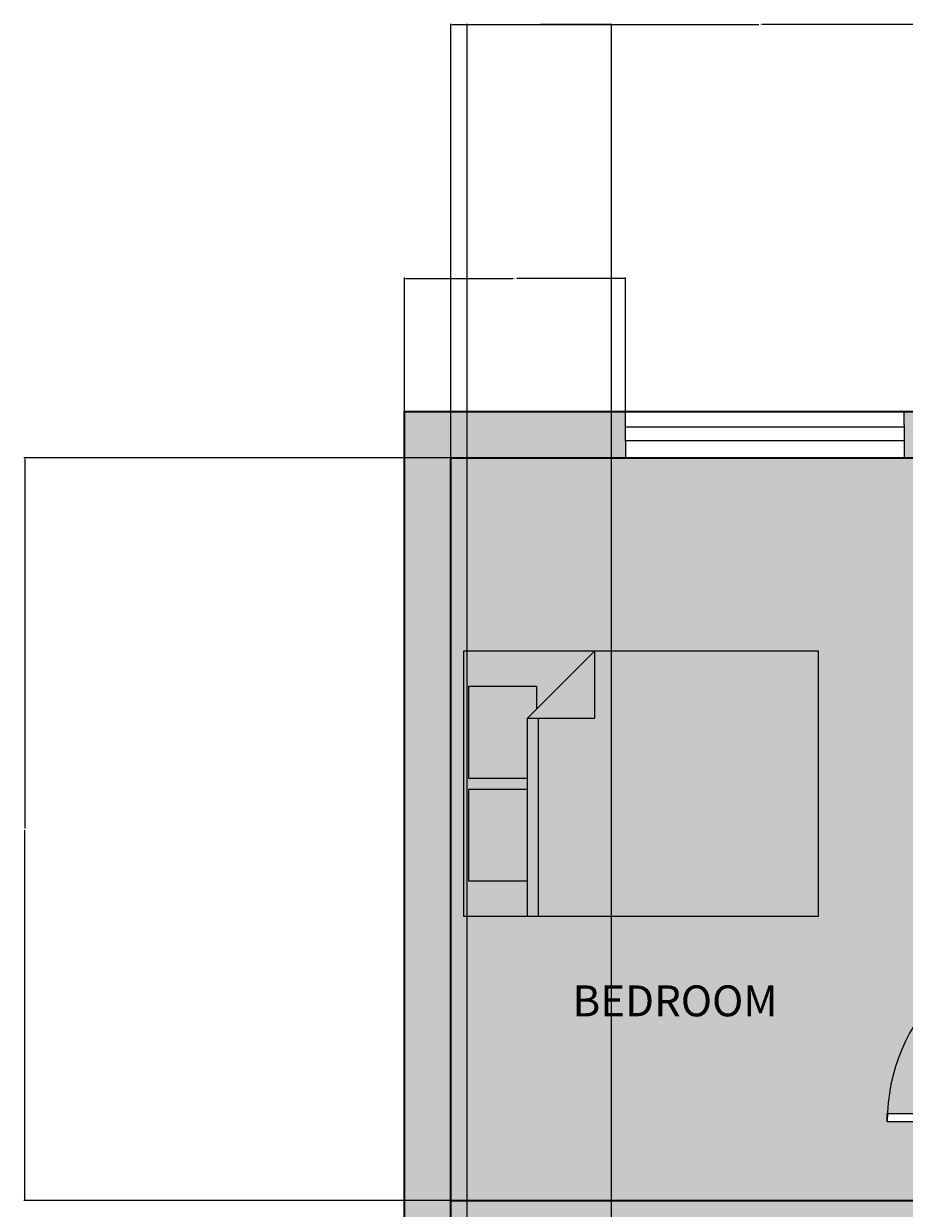
# Model space of a CAD drawing. Units: inches. Extents: x 3024 to 3952, y 1308 to 1863.
# Tile 22 of 29: x 3024 to 3195, y 1633 to 1863. Entities that reach past the tile are written whole.
import ezdxf

# ---------------------------------------------------------------- set-up
doc = ezdxf.new("R2010")
doc.units = ezdxf.units.IN
for name, color, linetype, lineweight in [('A-ANNO-DIMS', 2, 'Continuous', 18), ('A-AREA-IDEN', 7, 'Continuous', 18), ('A-DOOR', 4, 'Continuous', 18), ('A-FLOR-TILE-PATT', 7, 'Continuous', 13), ('A-FURN', 8, 'Continuous', 18), ('A-FURN-PATT', 9, 'Continuous', 13), ('A-GLAZ', 4, 'Continuous', 18), ('A-WALL', 7, 'Continuous', 35)]:
    doc.layers.add(name, color=color, linetype=linetype, lineweight=lineweight)
doc.layers.add('A-FLOR-PATT', color=254, linetype='Continuous', lineweight=13, true_color=0xfeeab9)
doc.layers.add('A-WALL-PATT', color=254, linetype='Continuous', lineweight=13, true_color=0xcecce6)
doc.styles.get("Standard").update_dxf_attribs({"font": 'arial.ttf'})
doc.dimstyles.get("Standard").update_dxf_attribs({"dimtxt": 0.18, "dimasz": 0.18, "dimexe": 0.18, "dimexo": 0.0625, "dimgap": 0.09, "dimtad": 0, "dimtih": 1, "dimtoh": 1, "dimdec": 4, "dimzin": 0, "dimdsep": 46, "dimtxsty": 'Standard', "dimcen": 0.09, "dimadec": 0, "dimazin": 0, "dimtfac": 1, "dimtdec": 4, "dimtofl": 0, "dimtmove": 0, "dimatfit": 3, "dimfxl": 1, "dimtolj": 1, "dimtzin": 0, "dimarcsym": 0})

# ---------------------------------------------------------------- blocks, each defined once
blk = doc.blocks.new('*U2')
for p, q in [((0, 0), (0, -6)), ((40, 0), (40, -6))]:
    blk.add_line(p, q)
blk.add_lwpolyline([(0, 0), (0, 40), (1.75, 40), (1.75, 0)], close=True)
blk.add_arc((0, 0), 40, 0, 90)
blk = doc.blocks.new('Bed - Queen')
for p, q in [((0, -80.00003), (0, 0)), ((0, 0), (59.99999, 0)), ((59.99999, 0), (59.99999, -80.00003)), ((7.99999, -1.2), (28.79998, -1.2)), ((7.99999, -14.4), (7.99999, -1.2)), ((28.79998, -1.2), (28.79998, -14.4)), ((31.19999, -1.2), (51.99999, -1.2)), ((31.19999, -14.4), (31.19999, -1.2)), ((51.99999, -1.2), (51.99999, -16.4)), ((0, -14.4), (44.8, -14.4)), ((59.99999, -29.6), (44.8, -14.4)), ((44.8, -14.4), (44.8, -29.6)), ((44.8, -16.8), (0, -16.8)), ((51.99999, -16.4), (46.79936, -16.4)), ((44.8, -29.6), (59.99999, -29.6)), ((59.99999, -80.00003), (0, -80.00003))]:
    blk.add_line(p, q)
blk = doc.blocks.new('WIN-BEDROOM-54IN')
for p, q in [((0, 5.99), (0, 9)), ((54.08, 6.41), (54.08, 9)), ((54.08, 6.41), (54.08, 5.99)), ((0, 3.28), (0, 0)), ((54.08, 3.69), (54.08, 0))]:
    blk.add_line(p, q)
blk.add_lwpolyline([(0, 5.99), (54.08, 5.99), (54.08, 3.28), (0, 3.28)], close=True)
blk = doc.blocks.new('*D38')
at = {"layer": 'A-ANNO-DIMS', "color": 0, "lineweight": -2, "transparency": 16777216}
for p, q in [((3106.76, 1778.67), (3106.76, 1862.78)), ((3226.76, 1778.67), (3226.76, 1862.78)), ((3106.94, 1862.6), (3166.48, 1862.6)), ((3226.58, 1862.6), (3167.04, 1862.6))]:
    blk.add_line(p, q, dxfattribs=at)
at = {"layer": 'A-ANNO-DIMS', "color": 0, "transparency": 16777216}
for points in [[(3106.94, 1862.63), (3106.94, 1862.57), (3106.76, 1862.6)], [(3226.58, 1862.63), (3226.58, 1862.57), (3226.76, 1862.6)]]:
    blk.add_solid(points, dxfattribs=at)
at = {"layer": 'Defpoints', "color": 0, "transparency": 16777216}
for p in [(3226.76, 1862.6), (3106.76, 1778.61), (3226.76, 1778.61)]:
    blk.add_point(p, dxfattribs=at)
at = {"layer": 'A-ANNO-DIMS', "color": 0, "transparency": 16777216, "insert": (3166.76, 1862.6), "char_height": 0.18, "attachment_point": 5}
blk.add_mtext('\\A1;120', dxfattribs=at)
blk = doc.blocks.new('*D42')
at = {"layer": 'A-ANNO-DIMS', "color": 0, "lineweight": -2, "transparency": 16777216}
for p, q in [((3106.7, 1778.61), (3023.95, 1778.61)), ((3024.13, 1778.43), (3024.13, 1706.79)), ((3024.13, 1634.79), (3024.13, 1706.43)), ((3106.7, 1634.61), (3023.95, 1634.61))]:
    blk.add_line(p, q, dxfattribs=at)
at = {"layer": 'A-ANNO-DIMS', "color": 0, "transparency": 16777216}
for points in [[(3024.1, 1778.43), (3024.16, 1778.43), (3024.13, 1778.61)], [(3024.1, 1634.79), (3024.16, 1634.79), (3024.13, 1634.61)]]:
    blk.add_solid(points, dxfattribs=at)
at = {"layer": 'Defpoints', "color": 0, "transparency": 16777216}
for p in [(3106.76, 1778.61), (3024.13, 1634.61), (3106.76, 1634.61)]:
    blk.add_point(p, dxfattribs=at)
at = {"layer": 'A-ANNO-DIMS', "color": 0, "transparency": 16777216, "insert": (3024.13, 1706.61), "char_height": 0.18, "attachment_point": 5}
blk.add_mtext('\\A1;144', dxfattribs=at)
blk = doc.blocks.new('*D71')
at = {"layer": 'A-ANNO-DIMS', "color": 0, "lineweight": -2, "transparency": 16777216}
for p, q in [((3097.76, 1787.67), (3097.76, 1813.56)), ((3097.94, 1813.38), (3118.78, 1813.38)), ((3140.42, 1813.38), (3119.58, 1813.38)), ((3140.6, 1787.67), (3140.6, 1813.56))]:
    blk.add_line(p, q, dxfattribs=at)
at = {"layer": 'A-ANNO-DIMS', "color": 0, "transparency": 16777216}
for points in [[(3097.94, 1813.41), (3097.94, 1813.35), (3097.76, 1813.38)], [(3140.42, 1813.41), (3140.42, 1813.35), (3140.6, 1813.38)]]:
    blk.add_solid(points, dxfattribs=at)
at = {"layer": 'Defpoints', "color": 0, "transparency": 16777216}
for p in [(3140.6, 1813.38), (3097.76, 1787.61), (3140.6, 1787.61)]:
    blk.add_point(p, dxfattribs=at)
at = {"layer": 'A-ANNO-DIMS', "color": 0, "transparency": 16777216, "insert": (3119.18, 1813.38), "char_height": 0.18, "attachment_point": 5}
blk.add_mtext('\\A1;42.83', dxfattribs=at)
blk = doc.blocks.new('*D80')
at = {"layer": 'A-ANNO-DIMS', "color": 0, "lineweight": -2, "transparency": 16777216}
for p, q in [((3109.9, 1617.34), (3109.9, 1862.78)), ((3137.9, 1606.84), (3137.9, 1862.78)), ((3110.08, 1862.6), (3123.68, 1862.6)), ((3137.72, 1862.6), (3124.12, 1862.6))]:
    blk.add_line(p, q, dxfattribs=at)
at = {"layer": 'A-ANNO-DIMS', "color": 0, "transparency": 16777216}
for points in [[(3110.08, 1862.63), (3110.08, 1862.57), (3109.9, 1862.6)], [(3137.72, 1862.63), (3137.72, 1862.57), (3137.9, 1862.6)]]:
    blk.add_solid(points, dxfattribs=at)
at = {"layer": 'Defpoints', "color": 0, "transparency": 16777216}
for p in [(3137.9, 1862.6), (3109.9, 1617.28), (3137.9, 1606.78)]:
    blk.add_point(p, dxfattribs=at)
at = {"layer": 'A-ANNO-DIMS', "color": 0, "transparency": 16777216, "insert": (3123.9, 1862.6), "char_height": 0.18, "attachment_point": 5}
blk.add_mtext('\\A1;28', dxfattribs=at)

msp = doc.modelspace()

# ---------------------------------------------------------------- hatches: boundary and pattern name
at = {"layer": 'A-FLOR-PATT', "transparency": 33554528}
h = msp.add_hatch(color=256, dxfattribs=at)
h.dxf.hatch_style = 1
h.paths.add_polyline_path([(3460.764, 1688.6064), (3412.764, 1688.6064), (3412.764, 1694.6064), (3460.764, 1694.6064), (3460.764, 1778.6064), (3406.764, 1778.6064), (3406.764, 1759.9514), (3318.2981, 1759.9514), (3318.2981, 1658.6064), (3322.5356, 1658.6064), (3322.5356, 1652.6064), (3292.764, 1652.6064), (3292.764, 1778.6064), (3106.764, 1778.6064), (3106.764, 1628.6064), (3172.764, 1628.6064), (3172.764, 1532.6064), (3166.764, 1532.6064), (3166.764, 1628.6064), (3106.764, 1628.6064), (3106.764, 1356.8452), (3202.812, 1356.8452), (3202.812, 1354.2534), (3202.812, 1353.8388), (3202.812, 1351.1212), (3202.812, 1347.8452), (3277.764, 1347.8452), (3277.764, 1353.8452), (3277.764, 1356.8452), (3277.764, 1442.6064), (3460.764, 1442.6064)])
h.paths.add_polyline_path([(3216.238, 1527.2064), (3216.238, 1491.2064), (3214.663, 1491.2064), (3214.663, 1491.2409, -0.39662236), (3180.243, 1526.6064), (3163.0285, 1526.6064), (3163.0285, 1531.1064), (3161.716, 1531.1064), (3161.716, 1561.1064), (3163.0285, 1561.1064), (3163.0285, 1531.1064), (3163.0285, 1526.6064), (3180.243, 1526.6064, 0.39662236), (3214.663, 1491.2409), (3214.663, 1527.2064)], flags=16)
h.paths.add_polyline_path([(3227.364, 1649.8972), (3191.364, 1649.8972), (3191.364, 1651.4722), (3227.364, 1651.4722)], flags=16)
h.paths.add_polyline_path([(3323.1172, 1606.7362), (3323.8545, 1606.8514), (3323.8545, 1594.8241), (3323.1172, 1594.9393)], flags=16)
h.paths.add_polyline_path([(3324.2232, 1606.909), (3330.1216, 1607.8307), (3330.1216, 1614.1093), (3339.3495, 1614.1093), (3340.2711, 1620.0078), (3352.4136, 1620.0078), (3353.3353, 1614.1093), (3359.9941, 1614.1093), (3360.9157, 1620.0078), (3373.0582, 1620.0078), (3373.9799, 1614.1093), (3383.2077, 1614.1093), (3383.2077, 1607.8307), (3389.1062, 1606.909), (3389.1062, 1594.7665), (3383.2077, 1593.8449), (3383.2077, 1587.5663), (3373.9799, 1587.5663), (3373.0583, 1581.6678), (3360.9157, 1581.6678), (3359.9941, 1587.5663), (3353.3353, 1587.5663), (3352.4136, 1581.6678), (3340.2711, 1581.6678), (3339.3495, 1587.5663), (3330.1216, 1587.5663), (3330.1216, 1593.8449), (3324.2232, 1594.7665)], flags=16)
h.paths.add_polyline_path([(3236.1584, 1693.1064), (3236.1584, 1723.1064), (3237.4709, 1723.1064), (3237.4709, 1693.1064)], flags=16)
h.paths.add_polyline_path([(3373.2158, 1600.6847), (3373.7965, 1600.7303), (3374.3268, 1600.7874), (3374.8132, 1600.8531), (3375.2621, 1600.9247), (3375.6801, 1600.9991), (3376.0736, 1601.0735), (3376.6855, 1601.19), (3377.366, 1601.3023), (3378.0667, 1601.3814), (3378.8026, 1601.4123), (3379.5865, 1601.3839), (3380.4537, 1601.2948), (3381.301, 1601.1717), (3382.0317, 1601.0433), (3382.4398, 1600.9607), (3382.6252, 1600.9201), (3382.919, 1600.8507), (3382.9044, 1600.8531), (3382.842, 1600.8678), (3382.7541, 1600.8896), (3382.6252, 1600.9201), (3382.4398, 1600.9607), (3382.1868, 1601.0119), (3381.8738, 1601.0711), (3381.5125, 1601.1346), (3381.1149, 1601.1988), (3380.6928, 1601.2601), (3380.2581, 1601.3149), (3379.8226, 1601.3597), (3379.3984, 1601.3908), (3378.9944, 1601.4054), (3378.6092, 1601.4042), (3378.2384, 1601.3886), (3377.8777, 1601.36), (3377.5227, 1601.32), (3377.1691, 1601.2698), (3376.8127, 1601.211), (3376.4491, 1601.145), (3376.0736, 1601.0735), (3375.4177, 1600.9494), (3374.5542, 1600.8119), (3373.5044, 1600.6988)], flags=0)
h.paths.add_polyline_path([(3380.0253, 1596.7351), (3380.499, 1596.6659), (3380.9706, 1596.6119), (3381.4375, 1596.5791), (3381.8971, 1596.5736), (3382.5886, 1596.6167), (3382.7848, 1596.6692), (3382.1465, 1596.5706), (3381.236, 1596.5815), (3380.3199, 1596.6865)], flags=0)
h.paths.add_polyline_path([(3369.6414, 1603.9617), (3370.1589, 1604.0021), (3370.6218, 1604.0539), (3371.0335, 1604.1173), (3371.3978, 1604.1921), (3371.7181, 1604.2785), (3371.9984, 1604.3761), (3372.2441, 1604.483), (3372.4611, 1604.5972), (3372.655, 1604.7163), (3372.8317, 1604.8384), (3372.9968, 1604.9611), (3373.3703, 1605.2455), (3373.8426, 1605.5328), (3374.4624, 1605.7539), (3375.1058, 1605.8302), (3375.7221, 1605.8261), (3376.4109, 1605.76), (3377.1534, 1605.6376), (3377.8945, 1605.473), (3378.1382, 1605.409), (3377.7394, 1605.5074), (3377.3509, 1605.5937), (3376.9704, 1605.6677), (3376.5999, 1605.7288), (3376.2417, 1605.7762), (3375.8979, 1605.8092), (3375.5707, 1605.8271), (3375.2621, 1605.8291), (3374.9745, 1605.8146), (3374.7092, 1605.7832), (3374.4647, 1605.7359), (3374.239, 1605.6742), (3374.0298, 1605.5996), (3373.835, 1605.5134), (3373.6525, 1605.4171), (3373.4801, 1605.3123), (3373.3156, 1605.2002), (3373.1562, 1605.0825), (3372.7603, 1604.781), (3372.236, 1604.4588), (3371.5738, 1604.2283), (3370.8493, 1604.0794), (3369.9262, 1603.976)], flags=0)
h.paths.add_polyline_path([(3366.7533, 1606.5832), (3367.1713, 1606.5519), (3367.5378, 1606.5374), (3367.8568, 1606.5394), (3368.1325, 1606.5573), (3368.3694, 1606.5903), (3368.5717, 1606.6377), (3368.7438, 1606.6988), (3368.89, 1606.7728), (3369.0146, 1606.8591), (3369.121, 1606.9568), (3369.2094, 1607.0646), (3369.2792, 1607.181), (3369.3295, 1607.3046), (3369.3596, 1607.4339), (3369.3688, 1607.5676), (3369.3565, 1607.7042), (3369.3218, 1607.8422), (3369.2649, 1607.9804), (3369.1893, 1608.1187), (3369.0993, 1608.2569), (3368.9992, 1608.3952), (3368.8934, 1608.5334), (3368.7861, 1608.6717), (3368.6817, 1608.8099), (3368.4212, 1609.1804), (3368.2685, 1609.7106), (3368.4883, 1610.1814), (3369.0537, 1610.4604), (3369.6717, 1610.5097), (3370.2812, 1610.3612), (3370.4805, 1610.2968), (3370.1882, 1610.3839), (3369.9284, 1610.4472), (3369.6905, 1610.4842), (3369.4662, 1610.4933), (3369.2555, 1610.4765), (3369.0608, 1610.4367), (3368.884, 1610.3767), (3368.7274, 1610.2994), (3368.5931, 1610.2077), (3368.4833, 1610.1045), (3368.4002, 1609.9927), (3368.3451, 1609.8747), (3368.3166, 1609.7517), (3368.3127, 1609.6244), (3368.331, 1609.4935), (3368.3696, 1609.3597), (3368.4261, 1609.2237), (3368.4985, 1609.0863), (3368.5845, 1608.9482), (3368.6817, 1608.8099), (3368.7861, 1608.6717), (3368.8934, 1608.5334), (3368.9992, 1608.3952), (3369.0993, 1608.2569), (3369.3398, 1607.8876), (3369.3941, 1607.2896), (3368.9774, 1606.7817), (3368.3928, 1606.5742), (3367.7162, 1606.5303), (3367.0044, 1606.5585)], flags=0)
h.paths.add_polyline_path([(3362.1859, 1610.2589), (3362.5478, 1610.2845), (3362.8348, 1610.3275), (3363.0585, 1610.3863), (3363.2303, 1610.4595), (3363.3619, 1610.5457), (3363.463, 1610.6432), (3363.5376, 1610.7502), (3363.5876, 1610.8643), (3363.6153, 1610.9834), (3363.6229, 1611.1055), (3363.6125, 1611.2283), (3363.5861, 1611.3496), (3363.5462, 1611.4673), (3363.4949, 1611.5797), (3363.4358, 1611.6871), (3363.3723, 1611.7902), (3363.3081, 1611.8897), (3363.2468, 1611.9863), (3363.192, 1612.0808), (3363.0258, 1612.4261), (3363.3371, 1612.8672), (3363.9008, 1612.9782), (3364.4822, 1612.9641), (3365.1098, 1612.9074), (3365.328, 1612.8805), (3364.9615, 1612.9208), (3364.6426, 1612.9496), (3364.3668, 1612.9669), (3364.1299, 1612.9726), (3363.9276, 1612.9669), (3363.7555, 1612.9496), (3363.6093, 1612.9208), (3363.4848, 1612.8805), (3363.3782, 1612.8289), (3363.2889, 1612.7672), (3363.2169, 1612.6969), (3363.1622, 1612.6193), (3363.1247, 1612.5361), (3363.1046, 1612.4484), (3363.1017, 1612.358), (3363.1161, 1612.266), (3363.1472, 1612.1738), (3363.192, 1612.0808), (3363.2468, 1611.9863), (3363.3081, 1611.8897), (3363.3723, 1611.7902), (3363.4358, 1611.6871), (3363.6363, 1611.323), (3363.5979, 1610.7003), (3363.0863, 1610.3651), (3362.3983, 1610.2622)], flags=0)
h.paths.add_polyline_path([(3352.356, 1581.2991), (3352.2408, 1580.5618), (3340.4439, 1580.5618), (3340.3287, 1581.2991)], flags=16)
h.paths.add_polyline_path([(3340.4439, 1621.1137), (3352.2408, 1621.1137), (3352.356, 1620.3764), (3340.3287, 1620.3764)], flags=16)
h.paths.add_polyline_path([(3278.4282, 1504.7424), (3290.3831, 1504.7424), (3290.3831, 1502.7499), (3291.0473, 1502.7499), (3291.0473, 1494.7799), (3290.3831, 1494.7799), (3290.3831, 1494.1158), (3291.0473, 1494.1158), (3291.0473, 1486.1458), (3290.3831, 1486.1458), (3290.3831, 1484.1533), (3291.0473, 1484.1533), (3291.0473, 1483.4892, -0.09090909), (3291.0473, 1468.8776), (3291.0473, 1468.2135), (3290.3831, 1468.2135), (3290.3831, 1464.8926), (3278.4282, 1464.8926), (3278.4282, 1472.8626), (3277.764, 1473.5268), (3277.764, 1478.84), (3278.4282, 1479.5042)], flags=16)
h.paths.add_polyline_path([(3278.7603, 1504.4103), (3290.051, 1504.4103), (3290.051, 1465.2247), (3278.7603, 1465.2247)], flags=0)
h.paths.add_polyline_path([(3123.904, 1600.7821), (3117.9039, 1602.7821), (3117.9039, 1599.7821), (3119.4039, 1599.7821), (3119.4039, 1596.7821), (3118.4039, 1596.7821), (3118.4039, 1598.7821), (3117.9039, 1598.7821), (3117.9039, 1596.2821), (3109.9039, 1596.2821), (3109.9039, 1617.2821), (3117.9039, 1617.2821), (3117.9039, 1610.7821), (3123.9038, 1612.7821, -0.70257121), (3137.9039, 1606.7822, -0.70256205)], flags=16)
h.paths.add_polyline_path([(3123.9039, 1602.7822), (3123.9039, 1610.7822, -0.73453329), (3136.9039, 1606.7822, -0.73452973)], flags=0)
h.paths.add_polyline_path([(3177.972, 1689.6473), (3109.2405, 1689.6473), (3109.2405, 1741.1959), (3177.972, 1741.1959)], flags=16)
h.paths.add_polyline_path([(3373.0006, 1581.2991), (3372.8854, 1580.5618), (3361.0885, 1580.5618), (3360.9733, 1581.2991)], flags=16)
h.paths.add_polyline_path([(3361.0885, 1621.1137), (3372.8854, 1621.1137), (3373.0006, 1620.3764), (3360.9733, 1620.3764)], flags=16)
h.paths.add_polyline_path([(3116.9039, 1598.2821, -0.41421356), (3116.1539, 1597.2821), (3111.9039, 1597.2821, -0.41421356), (3110.9039, 1598.0321), (3110.9039, 1615.2821, -0.41421356), (3111.6539, 1616.2821), (3115.9039, 1616.2821, -0.41421356), (3116.9039, 1615.5321)], flags=0)
h.paths.add_polyline_path([(3121.6122, 1728.1369), (3121.6122, 1696.5205), (3110.2715, 1696.5205), (3110.2715, 1714.3906), (3121.6122, 1714.3906), (3121.6122, 1716.4526), (3110.2715, 1716.4526), (3110.2715, 1734.3228), (3123.3304, 1734.3228), (3123.3304, 1729.8552), (3134.6711, 1741.1959), (3134.6711, 1728.1369)], flags=0)
h.paths.add_polyline_path([(3389.4748, 1606.8514), (3390.2122, 1606.7362), (3390.2122, 1594.9393), (3389.4748, 1594.8241)], flags=16)
h.paths.add_polyline_path([(3257.6842, 1762.8281), (3259.6842, 1768.8281), (3256.6842, 1768.8281), (3256.6842, 1767.3281), (3253.6842, 1767.3281), (3253.6842, 1768.3281), (3255.6842, 1768.3281), (3255.6842, 1768.8281), (3253.1842, 1768.8281), (3253.1842, 1776.8281), (3274.1842, 1776.8281), (3274.1842, 1768.8281), (3267.6842, 1768.8281), (3269.6842, 1762.8282, -0.70257121), (3263.6843, 1748.8282, -0.70256205)], flags=16)
h.paths.add_polyline_path([(3259.6842, 1762.8281), (3267.6843, 1762.8281, -0.73453329), (3263.6842, 1749.8282, -0.73452973)], flags=0)
h.paths.add_polyline_path([(3411.264, 1715.6064), (3411.264, 1716.9189), (3441.264, 1716.9189), (3441.264, 1715.6064)], flags=16)
h.paths.add_polyline_path([(3178.3806, 1449.1876), (3178.3806, 1397.639), (3109.6491, 1397.639), (3109.6491, 1449.1876)], flags=16)
h.paths.add_polyline_path([(3397.1501, 1541.7146), (3419.6183, 1541.7146), (3419.6183, 1496.7783), (3397.1501, 1496.7783)], flags=16)
h.paths.add_polyline_path([(3254.1842, 1770.5781), (3254.1842, 1774.8281, -0.41421356), (3254.9342, 1775.8281), (3272.1842, 1775.8281, -0.41421356), (3273.1842, 1775.0781), (3273.1842, 1770.8281, -0.41421356), (3272.4342, 1769.8281), (3255.1842, 1769.8281, -0.41421356)], flags=0)
h.paths.add_polyline_path([(3403.672, 1500.7601), (3403.6016, 1500.3997), (3403.5328, 1500.0441), (3403.4662, 1499.6867), (3403.4027, 1499.3226), (3403.3464, 1498.9532), (3403.3025, 1498.5811), (3403.2759, 1498.2091), (3403.2714, 1497.8401), (3403.3064, 1497.2813), (3403.3491, 1497.1219), (3403.2689, 1497.6395), (3403.2778, 1498.3719), (3403.3635, 1499.0984), (3403.4889, 1499.8168), (3403.6016, 1500.3997), (3403.672, 1500.7601), (3403.744, 1501.1315), (3403.817, 1501.5205), (3403.891, 1501.9336), (3403.9656, 1502.3769), (3404.0404, 1502.8572), (3404.115, 1503.3786), (3404.2264, 1504.2311), (3404.2571, 1504.5223), (3404.1552, 1503.6598), (3404.0063, 1502.6193), (3403.8604, 1501.7518), (3403.744, 1501.1315)], flags=0)
h.paths.add_polyline_path([(3406.5868, 1505.0416), (3406.6121, 1504.5236), (3406.6492, 1504.0526), (3406.6956, 1503.624), (3406.7491, 1503.2333), (3406.8072, 1502.8759), (3406.8676, 1502.5473), (3406.9281, 1502.243), (3407.0268, 1501.7597), (3407.1416, 1501.1368), (3407.2087, 1500.3904), (3407.1804, 1499.6703), (3407.1078, 1498.9956), (3407.0074, 1498.3199), (3406.8809, 1497.6059), (3406.7403, 1496.9627), (3406.7418, 1496.9824), (3406.7491, 1497.0249), (3406.8229, 1497.3409), (3406.8364, 1497.4025), (3406.878, 1497.6078), (3406.9261, 1497.8614), (3406.9777, 1498.1526), (3407.0298, 1498.4712), (3407.0797, 1498.8068), (3407.1243, 1499.149), (3407.1607, 1499.4874), (3407.1859, 1499.8115), (3407.1978, 1500.1137), (3407.1969, 1500.3962), (3407.1841, 1500.6642), (3407.1609, 1500.9225), (3407.1284, 1501.1761), (3407.0876, 1501.43), (3407.0398, 1501.6891), (3406.9862, 1501.9585), (3406.8832, 1502.4628), (3406.7712, 1503.0713), (3406.6657, 1503.8424), (3406.5924, 1504.7735)], flags=0)
h.paths.add_polyline_path([(3409.2517, 1507.8962), (3409.2752, 1507.4282), (3409.3079, 1507.0076), (3409.3501, 1506.6314), (3409.4015, 1506.2969), (3409.4624, 1506.0009), (3409.5326, 1505.7406), (3409.6119, 1505.5128), (3409.6988, 1505.3131), (3409.7915, 1505.1368), (3409.8883, 1504.9792), (3409.9875, 1504.8356), (3410.0872, 1504.7015), (3410.1859, 1504.572), (3410.4508, 1504.2132), (3410.7205, 1503.6035), (3410.8059, 1502.8824), (3410.7619, 1502.0875), (3410.6122, 1501.2299), (3410.4402, 1500.6169), (3410.2538, 1500.0031), (3410.0536, 1499.3219), (3409.9909, 1499.0812), (3410.1761, 1499.7472), (3410.3596, 1500.3513), (3410.4512, 1500.6561), (3410.5312, 1500.9412), (3410.6013, 1501.226), (3410.6614, 1501.512), (3410.7111, 1501.7964), (3410.7496, 1502.0763), (3410.7764, 1502.3489), (3410.7909, 1502.6114), (3410.7926, 1502.8608), (3410.7808, 1503.0944), (3410.7553, 1503.31), (3410.7169, 1503.5087), (3410.6667, 1503.6921), (3410.6061, 1503.8621), (3410.5361, 1504.0203), (3410.4578, 1504.1686), (3410.3726, 1504.3088), (3410.2815, 1504.4424), (3410.1859, 1504.572), (3410.0872, 1504.7015), (3409.859, 1505.0083), (3409.5943, 1505.5117), (3409.4266, 1506.1336), (3409.324, 1506.8011), (3409.2586, 1507.6407)], flags=0)
h.paths.add_polyline_path([(3411.4914, 1510.5878), (3411.4432, 1510.1586), (3411.4054, 1509.775), (3411.38, 1509.4354), (3411.3681, 1509.1376), (3411.3698, 1508.8784), (3411.3843, 1508.6542), (3411.4112, 1508.4618), (3411.4497, 1508.2974), (3411.4994, 1508.1575), (3411.5595, 1508.0388), (3411.6296, 1507.9375), (3411.7097, 1507.851), (3411.802, 1507.7792), (3411.9096, 1507.7225), (3412.0353, 1507.6817), (3412.1821, 1507.6572), (3412.3528, 1507.6496), (3412.5505, 1507.6597), (3412.778, 1507.6879), (3413.0364, 1507.7341), (3413.3194, 1507.7955), (3413.6188, 1507.8687), (3413.9264, 1507.95), (3414.234, 1508.036), (3414.5333, 1508.1232), (3414.8163, 1508.208), (3415.0747, 1508.287), (3415.3023, 1508.3569), (3415.5007, 1508.4158), (3415.6733, 1508.4617), (3416.1158, 1508.5538), (3416.512, 1508.2591), (3416.716, 1507.6581), (3416.61, 1507.0003), (3416.3052, 1506.3411), (3415.8928, 1505.618), (3415.7339, 1505.3633), (3415.9914, 1505.791), (3416.201, 1506.1583), (3416.3666, 1506.4739), (3416.4925, 1506.7462), (3416.5828, 1506.9838), (3416.6413, 1507.1949), (3416.6725, 1507.3883), (3416.6799, 1507.5705), (3416.6662, 1507.7417), (3416.6339, 1507.9), (3416.5851, 1508.0436), (3416.5223, 1508.1709), (3416.4478, 1508.28), (3416.3639, 1508.3692), (3416.273, 1508.4368), (3416.1765, 1508.4815), (3416.0718, 1508.5047), (3415.9553, 1508.5079), (3415.8237, 1508.493), (3415.6733, 1508.4617), (3415.5007, 1508.4158), (3415.3327, 1508.3659), (3414.6495, 1508.157), (3414.0606, 1507.9855), (3413.4456, 1507.8229), (3412.8838, 1507.701), (3412.5505, 1507.6597), (3412.0748, 1507.6354), (3411.595, 1507.8883), (3411.398, 1508.4429), (3411.3624, 1508.9927), (3411.3854, 1509.5711), (3411.4578, 1510.3071)], flags=0)
h.paths.add_polyline_path([(3135.0797, 1449.1876), (3135.0797, 1436.1286), (3122.0208, 1436.1286), (3122.0208, 1404.5122), (3110.6801, 1404.5122), (3110.6801, 1422.3823), (3122.0208, 1422.3823), (3122.0208, 1424.4443), (3110.6801, 1424.4443), (3110.6801, 1442.3145), (3123.739, 1442.3145), (3123.739, 1437.8469)], flags=0)
h.paths.add_polyline_path([(3416.4944, 1514.2949), (3416.4837, 1513.8511), (3416.4893, 1513.4867), (3416.5102, 1513.1926), (3416.5451, 1512.9593), (3416.5929, 1512.7775), (3416.6524, 1512.6379), (3416.7224, 1512.531), (3416.8017, 1512.4488), (3416.8886, 1512.3882), (3416.9813, 1512.3476), (3417.0781, 1512.3251), (3417.1773, 1512.3189), (3417.277, 1512.3274), (3417.3757, 1512.3488), (3417.4713, 1512.3813), (3417.5627, 1512.4229), (3417.65, 1512.471), (3417.7338, 1512.5225), (3417.8146, 1512.5747), (3417.8931, 1512.6245), (3417.9699, 1512.6691), (3418.2968, 1512.8265), (3418.6505, 1512.4645), (3418.7037, 1511.9342), (3418.6693, 1511.3839), (3418.6076, 1510.8228), (3418.5777, 1510.5927), (3418.6197, 1510.9333), (3418.6525, 1511.2311), (3418.6759, 1511.4903), (3418.6899, 1511.7144), (3418.6946, 1511.9069), (3418.6899, 1512.0713), (3418.6759, 1512.2112), (3418.6525, 1512.33), (3418.6197, 1512.4311), (3418.5778, 1512.5177), (3418.5276, 1512.5903), (3418.4705, 1512.6488), (3418.4075, 1512.6933), (3418.3399, 1512.7237), (3418.2686, 1512.7401), (3418.1951, 1512.7424), (3418.1204, 1512.7307), (3418.0455, 1512.7055), (3417.9792, 1512.6736), (3417.65, 1512.471), (3417.5627, 1512.4229), (3417.4713, 1512.3813), (3417.3757, 1512.3488), (3417.277, 1512.3274), (3416.878, 1512.2936), (3416.5757, 1512.7549), (3416.492, 1513.3145), (3416.4808, 1514.0384)], flags=0)
h.paths.add_polyline_path([(3392.8223, 1481.9454), (3396.7707, 1481.9454), (3396.7707, 1480.9201), (3428.3585, 1480.9201), (3428.3585, 1481.9454), (3432.3069, 1481.9454), (3432.3069, 1464.8354, -0.26666697), (3392.8223, 1464.8354)], flags=16)
h.paths.add_polyline_path([(3431.203, 1547.5428), (3450.8613, 1547.5428, -0.19047621), (3450.8614, 1484.031), (3431.203, 1484.031), (3431.203, 1488.5675), (3432.3809, 1488.5675), (3432.3809, 1543.0062), (3431.203, 1543.0062)], flags=16)
h.paths.add_polyline_path([(3451.9233, 1524.86, -0.04962821), (3451.9233, 1506.7138), (3446.7921, 1506.7138), (3446.7921, 1524.86)], flags=0)
h.paths.add_polyline_path([(3460.764, 1436.6064), (3277.764, 1436.6064), (3277.764, 1356.8452), (3277.764, 1353.8452), (3460.764, 1353.8452)], flags=17)
h.paths.add_polyline_path([(3121.3033, 1577.378), (3153.693, 1577.378), (3153.693, 1586.6752), (3121.3033, 1586.6752)], flags=24)
h.paths.add_polyline_path([(3164.1457, 1464.1276), (3210.4801, 1464.1276), (3210.4801, 1473.4247), (3164.1457, 1473.4247)], flags=24)
h.paths.add_polyline_path([(3343.1909, 1505.8863), (3373.7236, 1505.8863), (3373.7236, 1515.1773), (3343.1909, 1515.1773)], flags=24)
h.paths.add_polyline_path([(3337.6353, 1564.2926), (3370.0189, 1564.2926), (3370.0189, 1573.5836), (3337.6353, 1573.5836)], flags=24)
h.paths.add_polyline_path([(3419.204, 1753.8578), (3453.3997, 1753.8578), (3453.3997, 1762.9956), (3419.204, 1762.9956)], flags=24)
h.paths.add_polyline_path([(3341.2523, 1701.0246), (3381.0761, 1701.0246), (3381.0761, 1710.3156), (3341.2523, 1710.3156)], flags=24)
h.paths.add_polyline_path([(3245.8895, 1726.2997), (3278.2793, 1726.2997), (3278.2793, 1735.5968), (3245.8895, 1735.5968)], flags=24)
h.paths.add_polyline_path([(3128.8045, 1668.6736), (3175.1389, 1668.6736), (3175.1389, 1677.9707), (3128.8045, 1677.9707)], flags=24)
h.paths.add_polyline_path([(3345.9997, 1396.0062), (3389.09, 1396.0062), (3389.09, 1405.3033), (3345.9997, 1405.3033)], flags=24)
at = {"layer": 'A-FLOR-TILE-PATT', "transparency": 33554569}
h = msp.add_hatch(dxfattribs=at)
h.set_pattern_fill('ANGLE', color=256, scale=2)
h.set_pattern_definition([(0, (0, 0), (0, 13.97), [10.16, -3.81]), (90, (0, 0), (-13.97, 9e-16), [10.16, -3.81])])
h.paths.add_polyline_path([(3292.764, 1778.6064), (3232.764, 1778.6064), (3232.764, 1694.6064), (3236.1584, 1694.6064), (3236.1584, 1723.1064), (3237.4709, 1723.1064), (3237.4709, 1723.0777, -0.38700389), (3266.1209, 1694.6064), (3292.764, 1694.6064)])
h.paths.add_polyline_path([(3263.6843, 1748.8282, -0.70256205), (3257.6842, 1762.8281), (3259.6842, 1768.8281), (3256.6842, 1768.8281), (3256.6842, 1767.3281), (3253.6842, 1767.3281), (3253.6842, 1768.3281), (3255.6842, 1768.3281), (3255.6842, 1768.8281), (3253.1842, 1768.8281), (3253.1842, 1776.8281), (3274.1842, 1776.8281), (3274.1842, 1768.8281), (3267.6842, 1768.8281), (3269.6842, 1762.8282, -0.70257121)], flags=16)
h.paths.add_polyline_path([(3263.6842, 1749.8282, -0.73452973), (3259.6842, 1762.8281), (3267.6843, 1762.8281, -0.73453329)], flags=0)
h.paths.add_polyline_path([(3255.1842, 1769.8281, -0.41421356), (3254.1842, 1770.5781), (3254.1842, 1774.8281, -0.41421356), (3254.9342, 1775.8281), (3272.1842, 1775.8281, -0.41421356), (3273.1842, 1775.0781), (3273.1842, 1770.8281, -0.41421356), (3272.4342, 1769.8281)], flags=0)
h.paths.add_polyline_path([(3460.764, 1436.6064), (3277.764, 1436.6064), (3277.764, 1356.8452), (3277.764, 1353.8452), (3460.764, 1353.8452)])
h.paths.add_polyline_path([(3166.764, 1628.6064), (3106.764, 1628.6064), (3106.764, 1532.6064), (3133.066, 1532.6064, -0.38700389), (3161.716, 1561.0777), (3161.716, 1561.1064), (3163.0285, 1561.1064), (3163.0285, 1532.6064), (3166.764, 1532.6064)])
h.paths.add_polyline_path([(3123.904, 1600.7821), (3117.9039, 1602.7821), (3117.9039, 1599.7821), (3119.4039, 1599.7821), (3119.4039, 1596.7821), (3118.4039, 1596.7821), (3118.4039, 1598.7821), (3117.9039, 1598.7821), (3117.9039, 1596.2821), (3109.9039, 1596.2821), (3109.9039, 1617.2821), (3117.9039, 1617.2821), (3117.9039, 1610.7821), (3123.9038, 1612.7821, -0.70257121), (3137.9039, 1606.7822, -0.70256205)], flags=16)
h.paths.add_polyline_path([(3123.9039, 1602.7822), (3123.9039, 1610.7822, -0.73453329), (3136.9039, 1606.7822, -0.73452973)], flags=0)
h.paths.add_polyline_path([(3116.1539, 1597.2821), (3111.9039, 1597.2821, -0.41421356), (3110.9039, 1598.0321), (3110.9039, 1615.2821, -0.41421356), (3111.6539, 1616.2821), (3115.9039, 1616.2821, -0.41421356), (3116.9039, 1615.5321), (3116.9039, 1598.2821, -0.41421356)], flags=0)
h.paths.add_polyline_path([(3245.8895, 1726.2997), (3278.2793, 1726.2997), (3278.2793, 1735.5968), (3245.8895, 1735.5968)], flags=24)
h.paths.add_polyline_path([(3345.9997, 1396.0062), (3389.09, 1396.0062), (3389.09, 1405.3033), (3345.9997, 1405.3033)], flags=24)
h.paths.add_polyline_path([(3121.3033, 1577.378), (3153.693, 1577.378), (3153.693, 1586.6752), (3121.3033, 1586.6752)], flags=24)
at = {"layer": 'A-FURN-PATT'}
h = msp.add_hatch(color=256, dxfattribs=at)
h.dxf.hatch_style = 1
h.paths.add_polyline_path([(3134.6711, 1741.1959), (3109.2405, 1741.1959), (3109.2405, 1689.6473), (3121.6122, 1689.6473), (3121.6122, 1696.5205), (3110.2715, 1696.5205), (3110.2715, 1714.3906), (3121.6122, 1714.3906), (3121.6122, 1716.4526), (3110.2715, 1716.4526), (3110.2715, 1734.3228), (3123.3304, 1734.3228), (3123.3304, 1729.8552)])
h.paths.add_polyline_path([(3134.6711, 1741.1959), (3121.6122, 1728.1369), (3134.6711, 1728.1369)], flags=17)
h = msp.add_hatch(color=256, dxfattribs=at)
h.dxf.hatch_style = 1
h.paths.add_polyline_path([(3177.972, 1741.1959), (3134.6711, 1741.1959), (3134.6711, 1728.1369), (3123.6741, 1728.1369), (3123.6741, 1689.6473), (3177.972, 1689.6473)])
h = msp.add_hatch(color=256, dxfattribs=at)
h.dxf.hatch_style = 1
h.paths.add_polyline_path([(3121.6122, 1728.1369), (3123.3304, 1729.8552), (3123.3304, 1734.3228), (3110.2715, 1734.3228), (3110.2715, 1716.4526), (3121.6122, 1716.4526)])
h.paths.add_polyline_path([(3121.6122, 1714.3906), (3110.2715, 1714.3906), (3110.2715, 1696.5205), (3121.6122, 1696.5205)])
h = msp.add_hatch(color=256, dxfattribs=at)
h.dxf.hatch_style = 1
h.paths.add_polyline_path([(3123.6741, 1728.1369), (3121.6122, 1728.1369), (3121.6122, 1689.6473), (3123.6741, 1689.6473)])
at = {"layer": 'A-WALL-PATT'}
h = msp.add_hatch(color=256, dxfattribs=at)
h.dxf.hatch_style = 1
h.paths.add_polyline_path([(3106.764, 1778.6064), (3140.5977, 1778.6064), (3140.5977, 1781.8824), (3140.5977, 1784.6), (3140.5977, 1787.6064), (3097.764, 1787.6064), (3097.764, 1590.213), (3101.04, 1590.213), (3103.7576, 1590.213), (3106.764, 1590.213)])
h.paths.add_polyline_path([(3253.5314, 1781.8824), (3253.5314, 1784.6), (3253.5314, 1787.6064), (3194.6826, 1787.6064), (3194.6826, 1785.0146), (3194.6826, 1784.6), (3194.6826, 1781.8824), (3194.6826, 1778.6064), (3253.5314, 1778.6064)])
h.paths.add_polyline_path([(3333.856, 1782.2838), (3333.856, 1784.7474), (3333.856, 1787.6064), (3272.0523, 1787.6064), (3272.0523, 1785.0146), (3272.0523, 1784.6), (3272.0523, 1781.8824), (3272.0523, 1778.6064), (3333.856, 1778.6064)])
h.paths.add_polyline_path([(3428.8344, 1784.6), (3428.8344, 1787.6064), (3378.3947, 1787.6064), (3378.3947, 1784.7474), (3378.3947, 1782.2838), (3378.3947, 1778.6064), (3428.8344, 1778.6064), (3428.8344, 1781.8824)], flags=17)
h.paths.add_polyline_path([(3469.764, 1787.6064), (3451.9386, 1787.6064), (3451.9386, 1785.0146), (3451.9386, 1784.6), (3451.9386, 1781.8824), (3451.9386, 1778.6064), (3460.764, 1778.6064), (3460.764, 1353.8452), (3277.764, 1353.8452), (3277.764, 1347.8452), (3469.764, 1347.8452), (3469.764, 1353.8452)])
h.paths.add_polyline_path([(3106.764, 1571.6922), (3104.1722, 1571.6922), (3103.7576, 1571.6922), (3101.04, 1571.6922), (3097.764, 1571.6922), (3097.764, 1347.8452), (3148.7271, 1347.8452), (3148.7271, 1351.1212), (3148.7271, 1353.8388), (3148.7271, 1356.8452), (3106.764, 1356.8452)])
h.paths.add_polyline_path([(3277.764, 1532.6064), (3262.7605, 1532.6064), (3262.7605, 1582.9359), (3256.7605, 1582.9359), (3256.7605, 1532.6064), (3244.2116, 1532.6064), (3216.238, 1532.6064), (3216.238, 1527.2064), (3216.238, 1526.6064), (3271.764, 1526.6064), (3271.764, 1356.8452), (3202.812, 1356.8452), (3202.812, 1354.2534), (3202.812, 1353.8388), (3202.812, 1351.1212), (3202.812, 1347.8452), (3277.764, 1347.8452), (3277.764, 1353.8452), (3277.764, 1356.8452)])
h.paths.add_polyline_path([(3180.238, 1532.6064), (3163.0285, 1532.6064), (3163.0285, 1531.1064), (3163.0285, 1526.6064), (3180.243, 1526.6064, -0.00416688), (3180.238, 1527.2064)])
h.paths.add_polyline_path([(3133.0285, 1531.1064, -0.01250587), (3133.066, 1532.6064), (3106.764, 1532.6064), (3106.764, 1526.6064), (3133.0285, 1526.6064)], flags=17)
h.paths.add_polyline_path([(3172.764, 1628.6064), (3166.764, 1628.6064), (3166.764, 1532.6064), (3172.764, 1532.6064)])
h.paths.add_polyline_path([(3232.764, 1649.8972), (3227.364, 1649.8972), (3226.764, 1649.8972), (3226.764, 1634.6064), (3106.764, 1634.6064), (3106.764, 1628.6064), (3232.764, 1628.6064)])

# ---------------------------------------------------------------- linework, layer by layer
at = {"layer": 'A-WALL'}
for p, q in [((3097.764, 1787.6064), (3469.764, 1787.6064)), ((3097.764, 1347.8452), (3097.764, 1787.6064)), ((3106.764, 1778.6064), (3460.764, 1778.6064)), ((3106.764, 1356.8452), (3106.764, 1778.6064)), ((3106.764, 1634.6064), (3226.764, 1634.6064))]:
    msp.add_line(p, q, dxfattribs=at)

# ---------------------------------------------------------------- block references
at = {"layer": 'A-DOOR', "xscale": 0.9, "yscale": 0.9, "zscale": 0.9, "rotation": 90}
msp.add_blockref('*U2', (3227.364, 1649.8972), dxfattribs=at)
at = {"layer": 'A-FURN', "xscale": 0.8591429658128554, "yscale": 0.8591429658128554, "zscale": 0.8591429658128554, "rotation": 90}
msp.add_blockref('Bed - Queen', (3109.2405, 1689.6473), dxfattribs=at)
at = {"layer": 'A-GLAZ'}
msp.add_blockref('WIN-BEDROOM-54IN', (3140.598, 1778.606), dxfattribs=at)

# ---------------------------------------------------------------- texts
at = {"layer": 'A-AREA-IDEN'}
msp.add_text('BEDROOM', height=5.98971, dxfattribs=at).set_placement((3130.354, 1670.3253))

# ---------------------------------------------------------------- dimensions: what is measured, and where the dimension line sits
at = {"layer": 'A-ANNO-DIMS'}
for base, p1, p2, override, picture, middle in [((3226.764, 1862.6031), (3106.764, 1778.6064), (3226.764, 1778.6064), {"dimdec": 0, "dimlfac": 1, "dimrnd": 0, "dimzin": 0, "dimdsep": 46, "dimlunit": 2}, '*D38', (3166.764, 1862.6031)), ((3137.9039, 1862.6031), (3109.9039, 1617.2821), (3137.9039, 1606.7822), {"dimdec": 0, "dimlfac": 1, "dimrnd": 0, "dimzin": 0, "dimdsep": 46, "dimlunit": 2}, '*D80', (3123.9039, 1862.6031)), ((3140.5977, 1813.3814), (3097.764, 1787.6064), (3140.5977, 1787.6064), {"dimdec": 2, "dimlfac": 1, "dimrnd": 0, "dimzin": 0, "dimdsep": 46, "dimlunit": 2}, '*D71', (3119.1809, 1813.3814))]:
    dim = msp.add_linear_dim(base=base, p1=p1, p2=p2, dimstyle='Standard', override=override, dxfattribs=at)
    dim.commit()
    dim.dimension.update_dxf_attribs({"geometry": picture, "text_midpoint": middle})
dim = msp.add_linear_dim(base=(3024.1289, 1634.6064), p1=(3106.764, 1778.6064), p2=(3106.764, 1634.6064), angle=90, dimstyle='Standard', override={"dimdec": 0, "dimlfac": 1, "dimrnd": 0, "dimzin": 0, "dimdsep": 46, "dimlunit": 2}, dxfattribs=at)
dim.commit()
dim.dimension.update_dxf_attribs({"geometry": '*D42', "text_midpoint": (3024.1289, 1706.6064)})

doc.saveas('drawing.dxf')
